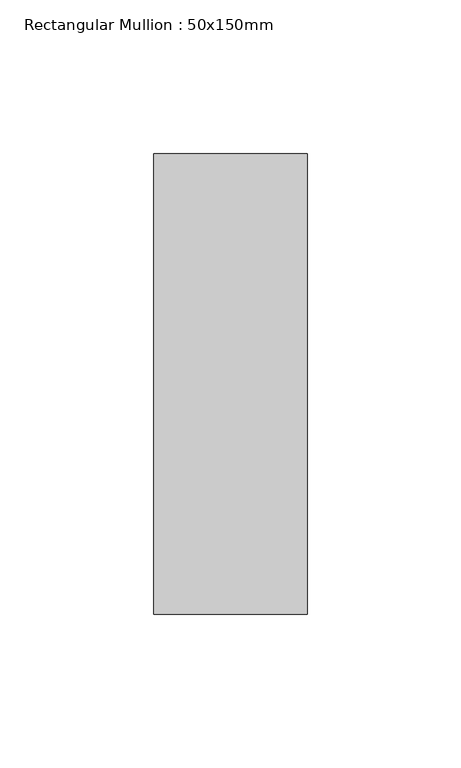
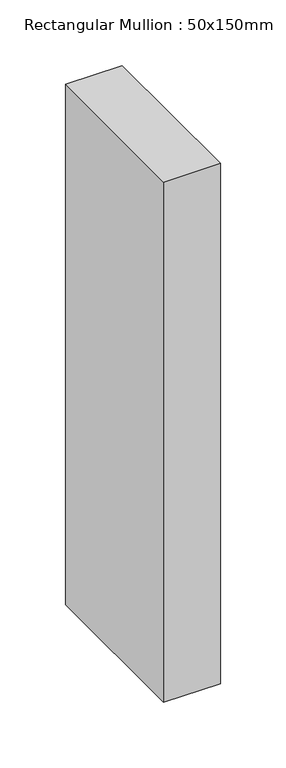
"""IFC4 building model written with IfcOpenShell, lengths in millimetres: member geometry, Rectangular Mullion : 50x150mm."""

from ifc_helpers import new_model, si_unit, frame, origin, place, context, project, spatial, polyline, outline, extrude, source, transform, mapped, element, save


def rectangular_mullion_50x150mm_e26dd5f5(model_context):
    return source(origin(), model_context, "Body", "SweptSolid", [
        extrude(outline(polyline([(25.0, 75.0), (25.0, -75.0), (-25.0, -75.0), (-25.0, 75.0), (25.0, 75.0)])), frame((0.0, 0.0, -484.2), z_axis=(0.0, 0.0, 1.0), x_axis=(1.0, 0.0, 0.0)), (0.0, 0.0, 1.0), 484.2),
    ])


if __name__ == "__main__":
    model = new_model("IFC4")
    model_context = context("Model", 3, world=origin())
    ifc_project = project(units=[si_unit("LENGTHUNIT", "METRE", prefix="MILLI")], contexts=[model_context])
    site = spatial("IfcSite", under=ifc_project)
    building = spatial("IfcBuilding", under=site)
    placement = place(None, origin())
    rectangular_mullion_50x150mm_shape = rectangular_mullion_50x150mm_e26dd5f5(model_context)
    element("IfcMember", 1, ObjectType="Rectangular Mullion : 50x150mm", at=placement, inside=building, context=model_context, shape_type="MappedRepresentation", body=[
        mapped(rectangular_mullion_50x150mm_shape, transform((0.0, 0.0, 0.0), x_axis=(1.0, 0.0, 0.0), y_axis=(0.0, 1.0, 0.0), z_axis=(0.0, 0.0, 1.0))),
    ])
    save(model, "model.ifc")

# Revit data of these elements
# Type "Rectangular Mullion : 50x150mm"
#   Keynote = "H11"
#   built-in parameter 1007304 = 0.492126 (stored number, unit not read)
#   built-in parameter 1007301 = 0.082021 (stored number, unit not read)
#   built-in parameter 1007300 = 0.082021 (stored number, unit not read)
# Element 1 (IfcMember, "Rectangular Mullion : 50x150mm")
#   Materials on its faces: "Aluminium"
# Materials
#   "Aluminium": class "Metal", colour RGB 247 247 247, transparency 0, Description = "Aluminium 6061", Cost = 0
